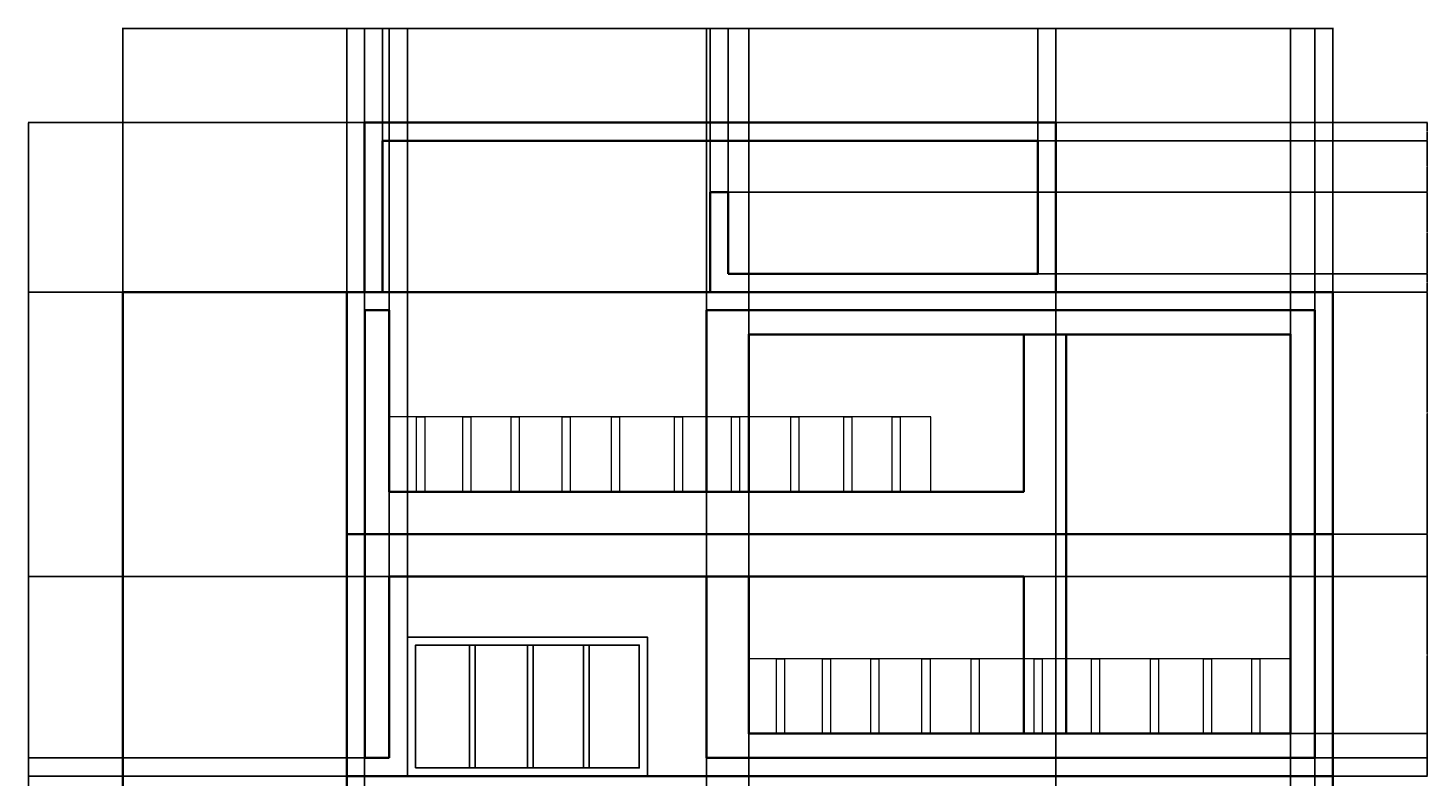
# Model space of a CAD drawing. Units: inches. Extents: x -26 to 668, y -42 to 976.
# Tile 3 of 3: x -26 to 668, y 605 to 976. Entities that reach past the tile are written whole.
import ezdxf

# ---------------------------------------------------------------- set-up
doc = ezdxf.new("R2010")
doc.units = ezdxf.units.IN
doc.header["$MEASUREMENT"] = 0
for name, color, linetype, lineweight in [('A-ANNO-DIMS', 2, 'Continuous', 18), ('A-ELEV', 7, 'Continuous', 35), ('A-FLOR-HRAL', 8, 'Continuous', 18), ('A-GLAZ', 4, 'Continuous', 25), ('A-ROOF', 7, 'Continuous', 35)]:
    doc.layers.add(name, color=color, linetype=linetype, lineweight=lineweight)
doc.styles.get("Standard").update_dxf_attribs({"font": 'arial.ttf'})
doc.dimstyles.get("Standard").update_dxf_attribs({"dimtxt": 0.18, "dimasz": 0.18, "dimexe": 0.18, "dimexo": 0.0625, "dimgap": 0.09, "dimtad": 0, "dimtih": 1, "dimtoh": 1, "dimdec": 4, "dimzin": 0, "dimdsep": 46, "dimtxsty": 'Standard', "dimcen": 0.09, "dimadec": 0, "dimazin": 0, "dimtfac": 1, "dimtdec": 4, "dimtofl": 0, "dimtmove": 0, "dimatfit": 3, "dimfxl": 1, "dimtolj": 1, "dimtzin": 0, "dimarcsym": 0})

# ---------------------------------------------------------------- blocks, each defined once
blk = doc.blocks.new('WIN-SLIDING-4P')
for p, q in [((192.66, 189.86), (192.66, 128.96)), ((195.46, 189.86), (195.46, 128.96)), ((221.46, 189.86), (221.46, 128.96)), ((224.25, 189.86), (224.25, 128.96)), ((249.2, 189.86), (249.2, 128.96)), ((251.99, 189.86), (251.99, 128.96))]:
    blk.add_line(p, q)
for points in [[(162.01, 124.96), (280.91, 124.96), (280.91, 193.86), (162.01, 193.86)], [(166.01, 128.96), (276.91, 128.96), (276.91, 189.86), (166.01, 189.86)]]:
    blk.add_lwpolyline(points, close=True)
blk = doc.blocks.new('RAILING-BALCONY')
for points in [[(331.17, 145.96), (599.79, 145.96), (599.79, 183.06), (331.17, 183.06)], [(344.86, 183.06), (348.85, 183.06), (348.85, 145.96), (344.86, 145.96)], [(367.74, 183.06), (371.72, 183.06), (371.72, 145.96), (367.74, 145.96)], [(391.66, 183.06), (395.64, 183.06), (395.64, 145.96), (391.66, 145.96)], [(417.04, 183.06), (421.03, 183.06), (421.03, 145.96), (417.04, 145.96)], [(441.38, 183.06), (445.37, 183.06), (445.37, 145.96), (441.38, 145.96)], [(472.69, 183.06), (476.68, 183.06), (476.68, 145.96), (472.69, 145.96)], [(501.02, 183.06), (505, 183.06), (505, 145.96), (501.02, 145.96)], [(530.39, 183.06), (534.38, 183.06), (534.38, 145.96), (530.39, 145.96)], [(556.62, 183.06), (560.61, 183.06), (560.61, 145.96), (556.62, 145.96)], [(580.54, 183.06), (584.53, 183.06), (584.53, 145.96), (580.54, 145.96)]]:
    blk.add_lwpolyline(points, close=True)
blk = doc.blocks.new('*D7')
at = {"layer": 'A-ANNO-DIMS', "color": 0, "lineweight": -2, "transparency": 16777216}
for p, q in [((20.79, 845.02), (20.79, 975.89)), ((20.97, 975.71), (320.51, 975.71)), ((620.61, 975.71), (321.08, 975.71)), ((620.79, 845.02), (620.79, 975.89))]:
    blk.add_line(p, q, dxfattribs=at)
at = {"layer": 'A-ANNO-DIMS', "color": 0, "transparency": 16777216}
for points in [[(20.97, 975.74), (20.97, 975.68), (20.79, 975.71)], [(620.61, 975.74), (620.61, 975.68), (620.79, 975.71)]]:
    blk.add_solid(points, dxfattribs=at)
at = {"layer": 'Defpoints', "color": 0, "transparency": 16777216}
for p in [(620.79, 975.71), (20.79, 844.96), (620.79, 844.96)]:
    blk.add_point(p, dxfattribs=at)
at = {"layer": 'A-ANNO-DIMS', "color": 0, "transparency": 16777216, "insert": (320.79, 975.71), "char_height": 0.18, "attachment_point": 5}
blk.add_mtext('\\A1;600', dxfattribs=at)
blk = doc.blocks.new('*D8')
at = {"layer": 'A-ANNO-DIMS', "color": 0, "lineweight": -2, "transparency": 16777216}
for p, q in [((140.59, 928.96), (-26.14, 928.96)), ((-25.96, 928.78), (-25.96, 467.14)), ((-25.96, 5.14), (-25.96, 466.78)), ((20.73, 4.96), (-26.14, 4.96))]:
    blk.add_line(p, q, dxfattribs=at)
at = {"layer": 'A-ANNO-DIMS', "color": 0, "transparency": 16777216}
for points in [[(-25.99, 928.78), (-25.93, 928.78), (-25.96, 928.96)], [(-25.99, 5.14), (-25.93, 5.14), (-25.96, 4.96)]]:
    blk.add_solid(points, dxfattribs=at)
at = {"layer": 'Defpoints', "color": 0, "transparency": 16777216}
for p in [(-25.96, 928.96), (140.65, 928.96), (20.79, 4.96)]:
    blk.add_point(p, dxfattribs=at)
at = {"layer": 'A-ANNO-DIMS', "color": 0, "transparency": 16777216, "insert": (-25.96, 466.96), "char_height": 0.18, "attachment_point": 5}
blk.add_mtext('\\A1;924', dxfattribs=at)
blk = doc.blocks.new('*D14')
at = {"layer": 'A-ANNO-DIMS', "color": 0, "lineweight": -2, "transparency": 16777216}
for p, q in [((620.86, 724.96), (667.72, 724.96)), ((667.54, 724.78), (667.54, 665.14)), ((667.54, 605.14), (667.54, 664.78)), ((620.86, 604.96), (667.72, 604.96))]:
    blk.add_line(p, q, dxfattribs=at)
at = {"layer": 'A-ANNO-DIMS', "color": 0, "transparency": 16777216}
for points in [[(667.51, 724.78), (667.57, 724.78), (667.54, 724.96)], [(667.51, 605.14), (667.57, 605.14), (667.54, 604.96)]]:
    blk.add_solid(points, dxfattribs=at)
at = {"layer": 'Defpoints', "color": 0, "transparency": 16777216}
for p in [(620.79, 724.96), (667.54, 724.96), (620.79, 604.96)]:
    blk.add_point(p, dxfattribs=at)
at = {"layer": 'A-ANNO-DIMS', "color": 0, "transparency": 16777216, "insert": (667.54, 664.96), "char_height": 0.18, "attachment_point": 5}
blk.add_mtext('\\A1;120', dxfattribs=at)
blk = doc.blocks.new('*D15')
at = {"layer": 'A-ANNO-DIMS', "color": 0, "lineweight": -2, "transparency": 16777216}
for p, q in [((620.86, 844.96), (667.72, 844.96)), ((667.54, 844.78), (667.54, 785.14)), ((667.54, 725.14), (667.54, 784.78)), ((620.86, 724.96), (667.72, 724.96))]:
    blk.add_line(p, q, dxfattribs=at)
at = {"layer": 'A-ANNO-DIMS', "color": 0, "transparency": 16777216}
for points in [[(667.51, 844.78), (667.57, 844.78), (667.54, 844.96)], [(667.51, 725.14), (667.57, 725.14), (667.54, 724.96)]]:
    blk.add_solid(points, dxfattribs=at)
at = {"layer": 'Defpoints', "color": 0, "transparency": 16777216}
for p in [(620.79, 844.96), (667.54, 844.96), (620.79, 724.96)]:
    blk.add_point(p, dxfattribs=at)
at = {"layer": 'A-ANNO-DIMS', "color": 0, "transparency": 16777216, "insert": (667.54, 784.96), "char_height": 0.18, "attachment_point": 5}
blk.add_mtext('\\A1;120', dxfattribs=at)
blk = doc.blocks.new('*D16')
at = {"layer": 'A-ANNO-DIMS', "color": 0, "lineweight": -2, "transparency": 16777216}
for p, q in [((131.83, 845.02), (131.83, 975.89)), ((132.01, 975.71), (135.85, 975.71)), ((140.47, 975.71), (136.64, 975.71)), ((140.65, 929.02), (140.65, 975.89))]:
    blk.add_line(p, q, dxfattribs=at)
at = {"layer": 'A-ANNO-DIMS', "color": 0, "transparency": 16777216}
for points in [[(132.01, 975.74), (132.01, 975.68), (131.83, 975.71)], [(140.47, 975.74), (140.47, 975.68), (140.65, 975.71)]]:
    blk.add_solid(points, dxfattribs=at)
at = {"layer": 'Defpoints', "color": 0, "transparency": 16777216}
for p in [(140.65, 975.71), (140.65, 928.96), (131.83, 844.96)]:
    blk.add_point(p, dxfattribs=at)
at = {"layer": 'A-ANNO-DIMS', "color": 0, "transparency": 16777216, "insert": (136.24, 975.71), "char_height": 0.18, "attachment_point": 5}
blk.add_mtext('\\A1;8.813', dxfattribs=at)
blk = doc.blocks.new('*D17')
at = {"layer": 'A-ANNO-DIMS', "color": 0, "lineweight": -2, "transparency": 16777216}
for p, q in [((140.65, 929.02), (140.65, 975.89)), ((140.83, 975.71), (145, 975.71)), ((149.47, 975.71), (145.3, 975.71)), ((149.65, 920.02), (149.65, 975.89))]:
    blk.add_line(p, q, dxfattribs=at)
at = {"layer": 'A-ANNO-DIMS', "color": 0, "transparency": 16777216}
for points in [[(140.83, 975.74), (140.83, 975.68), (140.65, 975.71)], [(149.47, 975.74), (149.47, 975.68), (149.65, 975.71)]]:
    blk.add_solid(points, dxfattribs=at)
at = {"layer": 'Defpoints', "color": 0, "transparency": 16777216}
for p in [(149.65, 975.71), (140.65, 928.96), (149.65, 919.96)]:
    blk.add_point(p, dxfattribs=at)
at = {"layer": 'A-ANNO-DIMS', "color": 0, "transparency": 16777216, "insert": (145.15, 975.71), "char_height": 0.18, "attachment_point": 5}
blk.add_mtext('\\A1;9', dxfattribs=at)
blk = doc.blocks.new('*D18')
at = {"layer": 'A-ANNO-DIMS', "color": 0, "lineweight": -2, "transparency": 16777216}
for p, q in [((149.65, 920.02), (149.65, 975.89)), ((149.83, 975.71), (230.46, 975.71)), ((311.86, 975.71), (231.23, 975.71)), ((312.04, 894.62), (312.04, 975.89))]:
    blk.add_line(p, q, dxfattribs=at)
at = {"layer": 'A-ANNO-DIMS', "color": 0, "transparency": 16777216}
for points in [[(149.83, 975.74), (149.83, 975.68), (149.65, 975.71)], [(311.86, 975.74), (311.86, 975.68), (312.04, 975.71)]]:
    blk.add_solid(points, dxfattribs=at)
at = {"layer": 'Defpoints', "color": 0, "transparency": 16777216}
for p in [(312.04, 975.71), (149.65, 919.96), (312.04, 894.55)]:
    blk.add_point(p, dxfattribs=at)
at = {"layer": 'A-ANNO-DIMS', "color": 0, "transparency": 16777216, "insert": (230.84, 975.71), "char_height": 0.18, "attachment_point": 5}
blk.add_mtext('\\A1;162.4', dxfattribs=at)
blk = doc.blocks.new('*D19')
at = {"layer": 'A-ANNO-DIMS', "color": 0, "lineweight": -2, "transparency": 16777216}
for p, q in [((312.04, 894.62), (312.04, 975.89)), ((312.22, 975.71), (316.39, 975.71)), ((320.86, 975.71), (316.69, 975.71)), ((321.04, 894.62), (321.04, 975.89))]:
    blk.add_line(p, q, dxfattribs=at)
at = {"layer": 'A-ANNO-DIMS', "color": 0, "transparency": 16777216}
for points in [[(312.22, 975.74), (312.22, 975.68), (312.04, 975.71)], [(320.86, 975.74), (320.86, 975.68), (321.04, 975.71)]]:
    blk.add_solid(points, dxfattribs=at)
at = {"layer": 'Defpoints', "color": 0, "transparency": 16777216}
for p in [(321.04, 975.71), (312.04, 894.55), (321.04, 894.55)]:
    blk.add_point(p, dxfattribs=at)
at = {"layer": 'A-ANNO-DIMS', "color": 0, "transparency": 16777216, "insert": (316.54, 975.71), "char_height": 0.18, "attachment_point": 5}
blk.add_mtext('\\A1;9', dxfattribs=at)
blk = doc.blocks.new('*D20')
at = {"layer": 'A-ANNO-DIMS', "color": 0, "lineweight": -2, "transparency": 16777216}
for p, q in [((321.04, 894.62), (321.04, 975.89)), ((321.22, 975.71), (397.35, 975.71)), ((474.25, 975.71), (398.12, 975.71)), ((474.43, 920.02), (474.43, 975.89))]:
    blk.add_line(p, q, dxfattribs=at)
at = {"layer": 'A-ANNO-DIMS', "color": 0, "transparency": 16777216}
for points in [[(321.22, 975.74), (321.22, 975.68), (321.04, 975.71)], [(474.25, 975.74), (474.25, 975.68), (474.43, 975.71)]]:
    blk.add_solid(points, dxfattribs=at)
at = {"layer": 'Defpoints', "color": 0, "transparency": 16777216}
for p in [(474.43, 975.71), (474.43, 919.96), (321.04, 894.55)]:
    blk.add_point(p, dxfattribs=at)
at = {"layer": 'A-ANNO-DIMS', "color": 0, "transparency": 16777216, "insert": (397.74, 975.71), "char_height": 0.18, "attachment_point": 5}
blk.add_mtext('\\A1;153.4', dxfattribs=at)
blk = doc.blocks.new('*D21')
at = {"layer": 'A-ANNO-DIMS', "color": 0, "lineweight": -2, "transparency": 16777216}
for p, q in [((474.43, 920.02), (474.43, 975.89)), ((474.61, 975.71), (478.78, 975.71)), ((483.25, 975.71), (479.08, 975.71)), ((483.43, 929.02), (483.43, 975.89))]:
    blk.add_line(p, q, dxfattribs=at)
at = {"layer": 'A-ANNO-DIMS', "color": 0, "transparency": 16777216}
for points in [[(474.61, 975.74), (474.61, 975.68), (474.43, 975.71)], [(483.25, 975.74), (483.25, 975.68), (483.43, 975.71)]]:
    blk.add_solid(points, dxfattribs=at)
at = {"layer": 'Defpoints', "color": 0, "transparency": 16777216}
for p in [(483.43, 975.71), (483.43, 928.96), (474.43, 919.96)]:
    blk.add_point(p, dxfattribs=at)
at = {"layer": 'A-ANNO-DIMS', "color": 0, "transparency": 16777216, "insert": (478.93, 975.71), "char_height": 0.18, "attachment_point": 5}
blk.add_mtext('\\A1;9', dxfattribs=at)
blk = doc.blocks.new('*D22')
at = {"layer": 'A-ANNO-DIMS', "color": 0, "lineweight": -2, "transparency": 16777216}
for p, q in [((140.65, 844.9), (140.65, -41.97)), ((483.43, 844.9), (483.43, -41.97)), ((140.83, -41.79), (311.65, -41.79)), ((483.25, -41.79), (312.43, -41.79))]:
    blk.add_line(p, q, dxfattribs=at)
at = {"layer": 'A-ANNO-DIMS', "color": 0, "transparency": 16777216}
for points in [[(140.83, -41.76), (140.83, -41.82), (140.65, -41.79)], [(483.25, -41.76), (483.25, -41.82), (483.43, -41.79)]]:
    blk.add_solid(points, dxfattribs=at)
at = {"layer": 'Defpoints', "color": 0, "transparency": 16777216}
for p in [(140.65, 844.96), (483.43, 844.96), (483.43, -41.79)]:
    blk.add_point(p, dxfattribs=at)
at = {"layer": 'A-ANNO-DIMS', "color": 0, "transparency": 16777216, "insert": (312.04, -41.79), "char_height": 0.18, "attachment_point": 5}
blk.add_mtext('\\A1;342.8', dxfattribs=at)
blk = doc.blocks.new('*D23')
at = {"layer": 'A-ANNO-DIMS', "color": 0, "lineweight": -2, "transparency": 16777216}
for p, q in [((321.1, 853.96), (667.72, 853.96)), ((667.54, 853.78), (667.54, 849.64)), ((667.54, 845.14), (667.54, 849.28)), ((483.49, 844.96), (667.72, 844.96))]:
    blk.add_line(p, q, dxfattribs=at)
at = {"layer": 'A-ANNO-DIMS', "color": 0, "transparency": 16777216}
for points in [[(667.51, 853.78), (667.57, 853.78), (667.54, 853.96)], [(667.51, 845.14), (667.57, 845.14), (667.54, 844.96)]]:
    blk.add_solid(points, dxfattribs=at)
at = {"layer": 'Defpoints', "color": 0, "transparency": 16777216}
for p in [(321.04, 853.96), (667.54, 853.96), (483.43, 844.96)]:
    blk.add_point(p, dxfattribs=at)
at = {"layer": 'A-ANNO-DIMS', "color": 0, "transparency": 16777216, "insert": (667.54, 849.46), "char_height": 0.18, "attachment_point": 5}
blk.add_mtext('\\A1;9', dxfattribs=at)
blk = doc.blocks.new('*D24')
at = {"layer": 'A-ANNO-DIMS', "color": 0, "lineweight": -2, "transparency": 16777216}
for p, q in [((312.1, 894.55), (667.72, 894.55)), ((667.54, 894.37), (667.54, 874.44)), ((667.54, 854.14), (667.54, 874.08)), ((321.1, 853.96), (667.72, 853.96))]:
    blk.add_line(p, q, dxfattribs=at)
at = {"layer": 'A-ANNO-DIMS', "color": 0, "transparency": 16777216}
for points in [[(667.51, 894.37), (667.57, 894.37), (667.54, 894.55)], [(667.51, 854.14), (667.57, 854.14), (667.54, 853.96)]]:
    blk.add_solid(points, dxfattribs=at)
at = {"layer": 'Defpoints', "color": 0, "transparency": 16777216}
for p in [(312.04, 894.55), (667.54, 894.55), (321.04, 853.96)]:
    blk.add_point(p, dxfattribs=at)
at = {"layer": 'A-ANNO-DIMS', "color": 0, "transparency": 16777216, "insert": (667.54, 874.26), "char_height": 0.18, "attachment_point": 5}
blk.add_mtext('\\A1;40.59', dxfattribs=at)
blk = doc.blocks.new('*D25')
at = {"layer": 'A-ANNO-DIMS', "color": 0, "lineweight": -2, "transparency": 16777216}
for p, q in [((474.49, 919.96), (667.72, 919.96)), ((667.54, 919.78), (667.54, 907.44)), ((667.54, 894.73), (667.54, 907.08)), ((312.1, 894.55), (667.72, 894.55))]:
    blk.add_line(p, q, dxfattribs=at)
at = {"layer": 'A-ANNO-DIMS', "color": 0, "transparency": 16777216}
for points in [[(667.51, 919.78), (667.57, 919.78), (667.54, 919.96)], [(667.51, 894.73), (667.57, 894.73), (667.54, 894.55)]]:
    blk.add_solid(points, dxfattribs=at)
at = {"layer": 'Defpoints', "color": 0, "transparency": 16777216}
for p in [(474.43, 919.96), (667.54, 919.96), (312.04, 894.55)]:
    blk.add_point(p, dxfattribs=at)
at = {"layer": 'A-ANNO-DIMS', "color": 0, "transparency": 16777216, "insert": (667.54, 907.26), "char_height": 0.18, "attachment_point": 5}
blk.add_mtext('\\A1;25.407', dxfattribs=at)
blk = doc.blocks.new('*D26')
at = {"layer": 'A-ANNO-DIMS', "color": 0, "lineweight": -2, "transparency": 16777216}
for p, q in [((483.49, 928.96), (667.72, 928.96)), ((667.54, 928.78), (667.54, 924.64)), ((667.54, 920.14), (667.54, 924.28)), ((474.49, 919.96), (667.72, 919.96))]:
    blk.add_line(p, q, dxfattribs=at)
at = {"layer": 'A-ANNO-DIMS', "color": 0, "transparency": 16777216}
for points in [[(667.51, 928.78), (667.57, 928.78), (667.54, 928.96)], [(667.51, 920.14), (667.57, 920.14), (667.54, 919.96)]]:
    blk.add_solid(points, dxfattribs=at)
at = {"layer": 'Defpoints', "color": 0, "transparency": 16777216}
for p in [(483.43, 928.96), (667.54, 928.96), (474.43, 919.96)]:
    blk.add_point(p, dxfattribs=at)
at = {"layer": 'A-ANNO-DIMS', "color": 0, "transparency": 16777216, "insert": (667.54, 924.46), "char_height": 0.18, "attachment_point": 5}
blk.add_mtext('\\A1;9', dxfattribs=at)
blk = doc.blocks.new('*D27')
at = {"layer": 'A-ANNO-DIMS', "color": 0, "lineweight": -2, "transparency": 16777216}
for p, q in [((140.59, 928.96), (-26.14, 928.96)), ((-25.96, 928.78), (-25.96, 887.14)), ((-25.96, 845.14), (-25.96, 886.78)), ((140.59, 844.96), (-26.14, 844.96))]:
    blk.add_line(p, q, dxfattribs=at)
at = {"layer": 'A-ANNO-DIMS', "color": 0, "transparency": 16777216}
for points in [[(-25.99, 928.78), (-25.93, 928.78), (-25.96, 928.96)], [(-25.99, 845.14), (-25.93, 845.14), (-25.96, 844.96)]]:
    blk.add_solid(points, dxfattribs=at)
at = {"layer": 'Defpoints', "color": 0, "transparency": 16777216}
for p in [(-25.96, 928.96), (140.65, 928.96), (140.65, 844.96)]:
    blk.add_point(p, dxfattribs=at)
at = {"layer": 'A-ANNO-DIMS', "color": 0, "transparency": 16777216, "insert": (-25.96, 886.96), "char_height": 0.18, "attachment_point": 5}
blk.add_mtext('\\A1;84', dxfattribs=at)
blk = doc.blocks.new('*D37')
at = {"layer": 'A-ANNO-DIMS', "color": 0, "lineweight": -2, "transparency": 16777216}
for p, q in [((152.83, 704.02), (152.83, 975.89)), ((153.01, 975.71), (157.03, 975.71)), ((161.83, 975.71), (157.82, 975.71)), ((162.01, 673.93), (162.01, 975.89))]:
    blk.add_line(p, q, dxfattribs=at)
at = {"layer": 'A-ANNO-DIMS', "color": 0, "transparency": 16777216}
for points in [[(153.01, 975.74), (153.01, 975.68), (152.83, 975.71)], [(161.83, 975.74), (161.83, 975.68), (162.01, 975.71)]]:
    blk.add_solid(points, dxfattribs=at)
at = {"layer": 'Defpoints', "color": 0, "transparency": 16777216}
for p in [(162.01, 975.71), (152.83, 703.96), (162.01, 673.86)]:
    blk.add_point(p, dxfattribs=at)
at = {"layer": 'A-ANNO-DIMS', "color": 0, "transparency": 16777216, "insert": (157.42, 975.71), "char_height": 0.18, "attachment_point": 5}
blk.add_mtext('\\A1;9.176', dxfattribs=at)
blk = doc.blocks.new('*D40')
at = {"layer": 'A-ANNO-DIMS', "color": 0, "lineweight": -2, "transparency": 16777216}
for p, q in [((140.77, 613.96), (-26.14, 613.96)), ((-25.96, 613.78), (-25.96, 609.64)), ((131.77, 604.96), (-26.14, 604.96)), ((-25.96, 605.14), (-25.96, 609.28))]:
    blk.add_line(p, q, dxfattribs=at)
at = {"layer": 'A-ANNO-DIMS', "color": 0, "transparency": 16777216}
for points in [[(-25.99, 613.78), (-25.93, 613.78), (-25.96, 613.96)], [(-25.99, 605.14), (-25.93, 605.14), (-25.96, 604.96)]]:
    blk.add_solid(points, dxfattribs=at)
at = {"layer": 'Defpoints', "color": 0, "transparency": 16777216}
for p in [(-25.96, 613.96), (140.83, 613.96), (131.83, 604.96)]:
    blk.add_point(p, dxfattribs=at)
at = {"layer": 'A-ANNO-DIMS', "color": 0, "transparency": 16777216, "insert": (-25.96, 609.46), "char_height": 0.18, "attachment_point": 5}
blk.add_mtext('\\A1;9', dxfattribs=at)
blk = doc.blocks.new('*D41')
at = {"layer": 'A-ANNO-DIMS', "color": 0, "lineweight": -2, "transparency": 16777216}
for p, q in [((152.77, 703.96), (-26.14, 703.96)), ((-25.96, 703.78), (-25.96, 659.14)), ((-25.96, 614.14), (-25.96, 658.78)), ((140.77, 613.96), (-26.14, 613.96))]:
    blk.add_line(p, q, dxfattribs=at)
at = {"layer": 'A-ANNO-DIMS', "color": 0, "transparency": 16777216}
for points in [[(-25.99, 703.78), (-25.93, 703.78), (-25.96, 703.96)], [(-25.99, 614.14), (-25.93, 614.14), (-25.96, 613.96)]]:
    blk.add_solid(points, dxfattribs=at)
at = {"layer": 'Defpoints', "color": 0, "transparency": 16777216}
for p in [(-25.96, 703.96), (152.83, 703.96), (140.83, 613.96)]:
    blk.add_point(p, dxfattribs=at)
at = {"layer": 'A-ANNO-DIMS', "color": 0, "transparency": 16777216, "insert": (-25.96, 658.96), "char_height": 0.18, "attachment_point": 5}
blk.add_mtext('\\A1;90', dxfattribs=at)
blk = doc.blocks.new('*D44')
at = {"layer": 'A-ANNO-DIMS', "color": 0, "lineweight": -2, "transparency": 16777216}
for p, q in [((611.86, 613.96), (667.72, 613.96)), ((667.54, 613.78), (667.54, 609.64)), ((620.86, 604.96), (667.72, 604.96)), ((667.54, 605.14), (667.54, 609.28))]:
    blk.add_line(p, q, dxfattribs=at)
at = {"layer": 'A-ANNO-DIMS', "color": 0, "transparency": 16777216}
for points in [[(667.51, 613.78), (667.57, 613.78), (667.54, 613.96)], [(667.51, 605.14), (667.57, 605.14), (667.54, 604.96)]]:
    blk.add_solid(points, dxfattribs=at)
at = {"layer": 'Defpoints', "color": 0, "transparency": 16777216}
for p in [(611.79, 613.96), (667.54, 613.96), (620.79, 604.96)]:
    blk.add_point(p, dxfattribs=at)
at = {"layer": 'A-ANNO-DIMS', "color": 0, "transparency": 16777216, "insert": (667.54, 609.46), "char_height": 0.18, "attachment_point": 5}
blk.add_mtext('\\A1;9', dxfattribs=at)
blk = doc.blocks.new('*D45')
at = {"layer": 'A-ANNO-DIMS', "color": 0, "lineweight": -2, "transparency": 16777216}
for p, q in [((599.86, 625.96), (667.72, 625.96)), ((667.54, 625.78), (667.54, 620.14)), ((667.54, 614.14), (667.54, 619.78)), ((611.86, 613.96), (667.72, 613.96))]:
    blk.add_line(p, q, dxfattribs=at)
at = {"layer": 'A-ANNO-DIMS', "color": 0, "transparency": 16777216}
for points in [[(667.51, 625.78), (667.57, 625.78), (667.54, 625.96)], [(667.51, 614.14), (667.57, 614.14), (667.54, 613.96)]]:
    blk.add_solid(points, dxfattribs=at)
at = {"layer": 'Defpoints', "color": 0, "transparency": 16777216}
for p in [(599.79, 625.96), (667.54, 625.96), (611.79, 613.96)]:
    blk.add_point(p, dxfattribs=at)
at = {"layer": 'A-ANNO-DIMS', "color": 0, "transparency": 16777216, "insert": (667.54, 619.96), "char_height": 0.18, "attachment_point": 5}
blk.add_mtext('\\A1;12', dxfattribs=at)
blk = doc.blocks.new('*D46')
at = {"layer": 'A-ANNO-DIMS', "color": 0, "lineweight": -2, "transparency": 16777216}
for p, q in [((467.57, 703.96), (667.72, 703.96)), ((667.54, 703.78), (667.54, 665.14)), ((667.54, 626.14), (667.54, 664.78)), ((599.86, 625.96), (667.72, 625.96))]:
    blk.add_line(p, q, dxfattribs=at)
at = {"layer": 'A-ANNO-DIMS', "color": 0, "transparency": 16777216}
for points in [[(667.51, 703.78), (667.57, 703.78), (667.54, 703.96)], [(667.51, 626.14), (667.57, 626.14), (667.54, 625.96)]]:
    blk.add_solid(points, dxfattribs=at)
at = {"layer": 'Defpoints', "color": 0, "transparency": 16777216}
for p in [(467.51, 703.96), (667.54, 703.96), (599.79, 625.96)]:
    blk.add_point(p, dxfattribs=at)
at = {"layer": 'A-ANNO-DIMS', "color": 0, "transparency": 16777216, "insert": (667.54, 664.96), "char_height": 0.18, "attachment_point": 5}
blk.add_mtext('\\A1;78', dxfattribs=at)
blk = doc.blocks.new('*D65')
at = {"layer": 'A-ANNO-DIMS', "color": 0, "lineweight": -2, "transparency": 16777216}
for p, q in [((20.79, 65.02), (20.79, 975.89)), ((20.97, 975.71), (75.86, 975.71)), ((131.65, 975.71), (76.77, 975.71)), ((131.83, 65.02), (131.83, 975.89))]:
    blk.add_line(p, q, dxfattribs=at)
at = {"layer": 'A-ANNO-DIMS', "color": 0, "transparency": 16777216}
for points in [[(20.97, 975.74), (20.97, 975.68), (20.79, 975.71)], [(131.65, 975.74), (131.65, 975.68), (131.83, 975.71)]]:
    blk.add_solid(points, dxfattribs=at)
at = {"layer": 'Defpoints', "color": 0, "transparency": 16777216}
for p in [(131.83, 975.71), (20.79, 64.96), (131.83, 64.96)]:
    blk.add_point(p, dxfattribs=at)
at = {"layer": 'A-ANNO-DIMS', "color": 0, "transparency": 16777216, "insert": (76.31, 975.71), "char_height": 0.18, "attachment_point": 5}
blk.add_mtext('\\A1;111.04', dxfattribs=at)
blk = doc.blocks.new('*D66')
at = {"layer": 'A-ANNO-DIMS', "color": 0, "lineweight": -2, "transparency": 16777216}
for p, q in [((310.17, 65.02), (310.17, 975.89)), ((310.35, 975.71), (320.47, 975.71)), ((330.99, 975.71), (320.87, 975.71)), ((331.17, 65.02), (331.17, 975.89))]:
    blk.add_line(p, q, dxfattribs=at)
at = {"layer": 'A-ANNO-DIMS', "color": 0, "transparency": 16777216}
for points in [[(310.35, 975.74), (310.35, 975.68), (310.17, 975.71)], [(330.99, 975.74), (330.99, 975.68), (331.17, 975.71)]]:
    blk.add_solid(points, dxfattribs=at)
at = {"layer": 'Defpoints', "color": 0, "transparency": 16777216}
for p in [(331.17, 975.71), (310.17, 64.96), (331.17, 64.96)]:
    blk.add_point(p, dxfattribs=at)
at = {"layer": 'A-ANNO-DIMS', "color": 0, "transparency": 16777216, "insert": (320.67, 975.71), "char_height": 0.18, "attachment_point": 5}
blk.add_mtext('\\A1;21', dxfattribs=at)
blk = doc.blocks.new('*D67')
at = {"layer": 'A-ANNO-DIMS', "color": 0, "lineweight": -2, "transparency": 16777216}
for p, q in [((331.17, 65.02), (331.17, 975.89)), ((331.35, 975.71), (465.09, 975.71)), ((599.61, 975.71), (465.88, 975.71)), ((599.79, 65.02), (599.79, 975.89))]:
    blk.add_line(p, q, dxfattribs=at)
at = {"layer": 'A-ANNO-DIMS', "color": 0, "transparency": 16777216}
for points in [[(331.35, 975.74), (331.35, 975.68), (331.17, 975.71)], [(599.61, 975.74), (599.61, 975.68), (599.79, 975.71)]]:
    blk.add_solid(points, dxfattribs=at)
at = {"layer": 'Defpoints', "color": 0, "transparency": 16777216}
for p in [(599.79, 975.71), (331.17, 64.96), (599.79, 64.96)]:
    blk.add_point(p, dxfattribs=at)
at = {"layer": 'A-ANNO-DIMS', "color": 0, "transparency": 16777216, "insert": (465.48, 975.71), "char_height": 0.18, "attachment_point": 5}
blk.add_mtext('\\A1;268.6', dxfattribs=at)
blk = doc.blocks.new('*D68')
at = {"layer": 'A-ANNO-DIMS', "color": 0, "lineweight": -2, "transparency": 16777216}
for p, q in [((599.79, 65.02), (599.79, 975.89)), ((599.97, 975.71), (605.58, 975.71)), ((611.61, 975.71), (606, 975.71)), ((611.79, 65.02), (611.79, 975.89))]:
    blk.add_line(p, q, dxfattribs=at)
at = {"layer": 'A-ANNO-DIMS', "color": 0, "transparency": 16777216}
for points in [[(599.97, 975.74), (599.97, 975.68), (599.79, 975.71)], [(611.61, 975.74), (611.61, 975.68), (611.79, 975.71)]]:
    blk.add_solid(points, dxfattribs=at)
at = {"layer": 'Defpoints', "color": 0, "transparency": 16777216}
for p in [(611.79, 975.71), (599.79, 64.96), (611.79, 64.96)]:
    blk.add_point(p, dxfattribs=at)
at = {"layer": 'A-ANNO-DIMS', "color": 0, "transparency": 16777216, "insert": (605.79, 975.71), "char_height": 0.18, "attachment_point": 5}
blk.add_mtext('\\A1;12', dxfattribs=at)
blk = doc.blocks.new('*D69')
at = {"layer": 'A-ANNO-DIMS', "color": 0, "lineweight": -2, "transparency": 16777216}
for p, q in [((611.79, 65.02), (611.79, 975.89)), ((611.97, 975.71), (616.15, 975.71)), ((620.61, 975.71), (616.44, 975.71)), ((620.79, 65.02), (620.79, 975.89))]:
    blk.add_line(p, q, dxfattribs=at)
at = {"layer": 'A-ANNO-DIMS', "color": 0, "transparency": 16777216}
for points in [[(611.97, 975.74), (611.97, 975.68), (611.79, 975.71)], [(620.61, 975.74), (620.61, 975.68), (620.79, 975.71)]]:
    blk.add_solid(points, dxfattribs=at)
at = {"layer": 'Defpoints', "color": 0, "transparency": 16777216}
for p in [(620.79, 975.71), (611.79, 64.96), (620.79, 64.96)]:
    blk.add_point(p, dxfattribs=at)
at = {"layer": 'A-ANNO-DIMS', "color": 0, "transparency": 16777216, "insert": (616.29, 975.71), "char_height": 0.18, "attachment_point": 5}
blk.add_mtext('\\A1;9', dxfattribs=at)

msp = doc.modelspace()

# ---------------------------------------------------------------- linework, layer by layer
at = {"layer": 'A-ELEV'}
for p, q in [((131.8349, 844.9609), (131.8349, 64.9609)), ((140.8349, 724.9609), (140.8349, 835.9609)), ((140.8349, 835.9609), (152.8349, 835.9609))]:
    msp.add_line(p, q, dxfattribs=at)
for points in [[(131.8349, 724.9609), (620.7944, 724.9609), (620.7944, 844.9609), (20.7944, 844.9609), (20.7944, 724.9609)], [(331.1714, 745.9609), (152.8349, 745.9609), (152.8349, 835.9609)], [(310.1714, 745.9609), (310.1714, 835.9609)], [(310.1714, 835.9609), (611.7944, 835.9609), (611.7944, 724.9609)], [(331.1714, 823.9609), (467.5079, 823.9609), (467.5079, 745.9609), (331.1714, 745.9609)], [(467.5079, 745.9609), (331.1714, 745.9609), (331.1714, 823.9609), (599.7944, 823.9609), (599.7944, 724.9609)], [(488.5079, 823.9609), (488.5079, 724.9609)], [(20.7944, 724.9609), (20.7944, 604.9609)], [(131.8349, 604.9609), (620.7944, 604.9609), (620.7944, 724.9609), (131.8349, 724.9609)], [(140.8349, 724.9609), (140.8349, 613.9609), (152.8349, 613.9609)], [(319.1714, 613.9609), (611.7944, 613.9609), (611.7944, 724.9609)], [(467.5079, 703.9609), (331.1714, 703.9609), (331.1714, 625.9609), (599.7944, 625.9609), (599.7944, 724.9609)], [(488.5079, 625.9609), (488.5079, 724.9609)], [(331.1714, 703.9609), (152.8349, 703.9609), (152.8349, 613.9609)], [(310.1714, 703.9609), (310.1714, 613.9609)], [(331.1714, 625.9609), (467.5079, 625.9609), (467.5079, 703.9609), (331.1714, 703.9609)], [(310.1714, 613.9609), (479.5079, 613.9609)], [(20.7944, 604.9609), (20.7944, 484.9609)], [(131.8349, 484.9609), (620.7944, 484.9609), (620.7944, 604.9609), (131.8349, 604.9609)]]:
    msp.add_lwpolyline(points, dxfattribs=at)
at = {"layer": 'A-ROOF'}
msp.add_lwpolyline([(140.6477, 844.9609), (483.4325, 844.9609), (483.4325, 928.9609), (140.6477, 928.9609)], close=True, dxfattribs=at)
for points in [[(321.0401, 853.9609), (474.4325, 853.9609), (474.4325, 919.9609), (149.6477, 919.9609), (149.6477, 844.9609)], [(321.0401, 853.9609), (321.0401, 894.5536), (312.0401, 894.5536), (312.0401, 844.9609)]]:
    msp.add_lwpolyline(points, dxfattribs=at)

# ---------------------------------------------------------------- block references
at = {"layer": 'A-FLOR-HRAL'}
for p in [(-178.3365, 600), (0, 480)]:
    msp.add_blockref('RAILING-BALCONY', p, dxfattribs=at)
at = {"layer": 'A-GLAZ'}
msp.add_blockref('WIN-SLIDING-4P', (0, 480), dxfattribs=at)

# ---------------------------------------------------------------- dimensions: what is measured, and where the dimension line sits
at = {"layer": 'A-ANNO-DIMS'}
for base, p1, p2, override, picture, middle in [((620.7944, 975.7109), (20.7944, 844.9609), (620.7944, 844.9609), {"dimdec": 0, "dimlfac": 1, "dimrnd": 0, "dimzin": 0, "dimdsep": 46, "dimlunit": 2}, '*D7', (320.7944, 975.7109)), ((131.8349, 975.7109), (20.7944, 64.9609), (131.8349, 64.9609), {"dimdec": 2, "dimlfac": 1, "dimrnd": 0, "dimzin": 0, "dimdsep": 46, "dimlunit": 2}, '*D65', (76.3146, 975.7109)), ((140.6477, 975.7109), (131.8349, 844.9609), (140.6477, 928.9609), {"dimdec": 3, "dimlfac": 1, "dimrnd": 0, "dimzin": 0, "dimdsep": 46, "dimlunit": 2}, '*D16', (136.2413, 975.7109)), ((149.6477, 975.7109), (140.6477, 928.9609), (149.6477, 919.9609), {"dimdec": 0, "dimlfac": 1, "dimrnd": 0, "dimzin": 0, "dimdsep": 46, "dimlunit": 2}, '*D17', (145.1477, 975.7109)), ((312.0401, 975.7109), (149.6477, 919.9609), (312.0401, 894.5536), {"dimdec": 1, "dimlfac": 1, "dimrnd": 0, "dimzin": 0, "dimdsep": 46, "dimlunit": 2}, '*D18', (230.8439, 975.7109)), ((162.0107, 975.7109), (152.8349, 703.9609), (162.0107, 673.8637), {"dimdec": 3, "dimlfac": 1, "dimrnd": 0, "dimzin": 0, "dimdsep": 46, "dimlunit": 2}, '*D37', (157.4228, 975.7109)), ((331.1714, 975.7109), (310.1714, 64.9609), (331.1714, 64.9609), {"dimdec": 0, "dimlfac": 1, "dimrnd": 0, "dimzin": 0, "dimdsep": 46, "dimlunit": 2}, '*D66', (320.6714, 975.7109)), ((321.0401, 975.7109), (312.0401, 894.5536), (321.0401, 894.5536), {"dimdec": 0, "dimlfac": 1, "dimrnd": 0, "dimzin": 0, "dimdsep": 46, "dimlunit": 2}, '*D19', (316.5401, 975.7109)), ((474.4325, 975.7109), (321.0401, 894.5536), (474.4325, 919.9609), {"dimdec": 1, "dimlfac": 1, "dimrnd": 0, "dimzin": 0, "dimdsep": 46, "dimlunit": 2}, '*D20', (397.7363, 975.7109)), ((599.7944, 975.7109), (331.1714, 64.9609), (599.7944, 64.9609), {"dimdec": 1, "dimlfac": 1, "dimrnd": 0, "dimzin": 0, "dimdsep": 46, "dimlunit": 2}, '*D67', (465.4829, 975.7109)), ((483.4325, 975.7109), (474.4325, 919.9609), (483.4325, 928.9609), {"dimdec": 0, "dimlfac": 1, "dimrnd": 0, "dimzin": 0, "dimdsep": 46, "dimlunit": 2}, '*D21', (478.9325, 975.7109)), ((611.7944, 975.7109), (599.7944, 64.9609), (611.7944, 64.9609), {"dimdec": 0, "dimlfac": 1, "dimrnd": 0, "dimzin": 0, "dimdsep": 46, "dimlunit": 2}, '*D68', (605.7944, 975.7109)), ((620.7944, 975.7109), (611.7944, 64.9609), (620.7944, 64.9609), {"dimdec": 0, "dimlfac": 1, "dimrnd": 0, "dimzin": 0, "dimdsep": 46, "dimlunit": 2}, '*D69', (616.2944, 975.7109)), ((483.4325, -41.7891), (140.6477, 844.9609), (483.4325, 844.9609), {"dimdec": 1, "dimlfac": 1, "dimrnd": 0, "dimzin": 0, "dimdsep": 46, "dimlunit": 2}, '*D22', (312.0401, -41.7891))]:
    dim = msp.add_linear_dim(base=base, p1=p1, p2=p2, dimstyle='Standard', override=override, dxfattribs=at)
    dim.commit()
    dim.dimension.update_dxf_attribs({"geometry": picture, "text_midpoint": middle})
for base, p1, p2, override, picture, middle in [((-25.9556, 928.9609), (20.7944, 4.9609), (140.6477, 928.9609), {"dimdec": 0, "dimlfac": 1, "dimrnd": 0, "dimzin": 0, "dimdsep": 46, "dimlunit": 2}, '*D8', (-25.9556, 466.9609)), ((-25.9556, 928.9609), (140.6477, 844.9609), (140.6477, 928.9609), {"dimdec": 0, "dimlfac": 1, "dimrnd": 0, "dimzin": 0, "dimdsep": 46, "dimlunit": 2}, '*D27', (-25.9556, 886.9609)), ((667.5444, 928.9609), (474.4325, 919.9609), (483.4325, 928.9609), {"dimdec": 0, "dimlfac": 1, "dimrnd": 0, "dimzin": 0, "dimdsep": 46, "dimlunit": 2}, '*D26', (667.5444, 924.4609)), ((667.5444, 919.9609), (312.0401, 894.5536), (474.4325, 919.9609), {"dimdec": 3, "dimlfac": 1, "dimrnd": 0, "dimzin": 0, "dimdsep": 46, "dimlunit": 2}, '*D25', (667.5444, 907.2573)), ((667.5444, 894.5536), (321.0401, 853.9609), (312.0401, 894.5536), {"dimdec": 2, "dimlfac": 1, "dimrnd": 0, "dimzin": 0, "dimdsep": 46, "dimlunit": 2}, '*D24', (667.5444, 874.2573)), ((667.5444, 853.9609), (483.4325, 844.9609), (321.0401, 853.9609), {"dimdec": 0, "dimlfac": 1, "dimrnd": 0, "dimzin": 0, "dimdsep": 46, "dimlunit": 2}, '*D23', (667.5444, 849.4609)), ((667.5444, 844.9609), (620.7944, 724.9609), (620.7944, 844.9609), {"dimdec": 0, "dimlfac": 1, "dimrnd": 0, "dimzin": 0, "dimdsep": 46, "dimlunit": 2}, '*D15', (667.5444, 784.9609)), ((667.5444, 724.9609), (620.7944, 604.9609), (620.7944, 724.9609), {"dimdec": 0, "dimlfac": 1, "dimrnd": 0, "dimzin": 0, "dimdsep": 46, "dimlunit": 2}, '*D14', (667.5444, 664.9609)), ((-25.9556, 703.9609), (140.8349, 613.9609), (152.8349, 703.9609), {"dimdec": 0, "dimlfac": 1, "dimrnd": 0, "dimzin": 0, "dimdsep": 46, "dimlunit": 2}, '*D41', (-25.9556, 658.9609)), ((667.5444, 703.9609), (599.7944, 625.9609), (467.5079, 703.9609), {"dimdec": 0, "dimlfac": 1, "dimrnd": 0, "dimzin": 0, "dimdsep": 46, "dimlunit": 2}, '*D46', (667.5444, 664.9609)), ((667.5444, 625.9609), (611.7944, 613.9609), (599.7944, 625.9609), {"dimdec": 0, "dimlfac": 1, "dimrnd": 0, "dimzin": 0, "dimdsep": 46, "dimlunit": 2}, '*D45', (667.5444, 619.9609)), ((-25.9556, 613.9609), (131.8349, 604.9609), (140.8349, 613.9609), {"dimdec": 0, "dimlfac": 1, "dimrnd": 0, "dimzin": 0, "dimdsep": 46, "dimlunit": 2}, '*D40', (-25.9556, 609.4609)), ((667.5444, 613.9609), (620.7944, 604.9609), (611.7944, 613.9609), {"dimdec": 0, "dimlfac": 1, "dimrnd": 0, "dimzin": 0, "dimdsep": 46, "dimlunit": 2}, '*D44', (667.5444, 609.4609))]:
    dim = msp.add_linear_dim(base=base, p1=p1, p2=p2, angle=90, dimstyle='Standard', override=override, dxfattribs=at)
    dim.commit()
    dim.dimension.update_dxf_attribs({"geometry": picture, "text_midpoint": middle})

doc.saveas('drawing.dxf')
